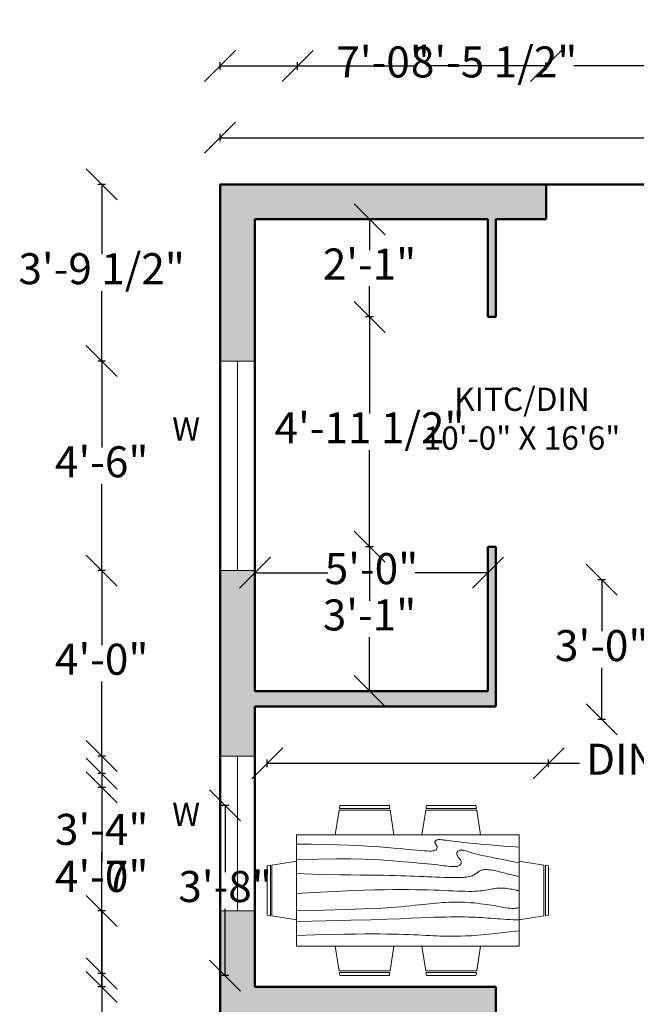
# Model space of a CAD drawing. Units: inches. Extents: x 3121 to 3511, y 1323 to 1998.
# Tile 9 of 10: x 3138 to 3297, y 1744 to 1998. Entities that reach past the tile are written whole.
import ezdxf

# ---------------------------------------------------------------- set-up
doc = ezdxf.new("R2010")
doc.units = ezdxf.units.IN
for name, color, linetype, lineweight in [('A-ANNO-DIMS', 2, 'Continuous', 18), ('A-ANNO-TEXT', 7, 'Continuous', 18), ('A-AREA-IDEN', 7, 'Continuous', 25), ('A-FURN', 8, 'Continuous', 18), ('A-GLAZ', 4, 'Continuous', 18), ('A-WALL', 7, 'Continuous', 50), ('A-WALL-PATT', 3, 'Continuous', 13)]:
    doc.layers.add(name, color=color, linetype=linetype, lineweight=lineweight)
doc.styles.get("Standard").update_dxf_attribs({"font": 'arial.ttf'})
doc.dimstyles.new('ISO-25', dxfattribs={"dimtxt": 8, "dimasz": 8, "dimexe": 1, "dimexo": 1, "dimtad": 0, "dimtih": 1, "dimtoh": 1, "dimlunit": 3, "dimtxsty": 'Standard', "dimblk": 'OBLIQUE', "dimcen": 2.5, "dimclrt": 1, "dimadec": 0, "dimazin": 0, "dimtfac": 1, "dimtmove": 0, "dimatfit": 3, "dimfxl": 1, "dimfxlon": 1, "dimarcsym": 0})

# ---------------------------------------------------------------- blocks, each defined once
blk = doc.blocks.new('Dining Set - 36 x 72 in.')
for p, q in [((-22.2343, 26.00059), (-23.4847, 17.99762)), ((-22.2304, 26), (-5.7608, 26)), ((-22, 27.5), (-22.1562, 26.50042)), ((-5.8416, 26.5), (-22.1534, 26.5)), ((-22, 27.5), (-6, 27.5)), ((-5.8437, 26.49966), (-6, 27.5)), ((-4.5152, 17.99762), (-5.7655, 25.99926)), ((5.7657, 26.00059), (4.5153, 17.99762)), ((5.7696, 26), (22.2392, 26)), ((6, 27.5), (5.8438, 26.50042)), ((22.1584, 26.5), (5.8466, 26.5)), ((6, 27.5), (22, 27.5)), ((22.1563, 26.49966), (22, 27.5)), ((23.4848, 17.99762), (22.2345, 25.99926)), ((36, 18), (-36, 18)), ((-36, 18), (-36, -18)), ((36, -18), (36, 18)), ((-45.5, 8), (-44.5004, 8.15617)), ((-45.5, 8), (-45.5, -8)), ((-44.5, -8.15843), (-44.5, 8.15338)), ((-44.0006, 8.23428), (-35.9976, 9.48474)), ((-44, 8.23041), (-44, -8.23915)), ((44.0006, 8.23428), (35.9976, 9.48474)), ((44, 8.23041), (44, -8.23915)), ((44.5, -8.15843), (44.5, 8.15338)), ((45.5, 8), (44.5005, 8.15617)), ((45.5, 8), (45.5, -8)), ((-44.4997, -8.15631), (-45.5, -8)), ((-35.9976, -9.48476), (-43.9993, -8.2345)), ((35.9976, -9.48476), (43.9993, -8.2345)), ((44.4997, -8.15631), (45.5, -8)), ((-36, -18), (36, -18)), ((-22.2343, -26.0006), (-23.4847, -17.99762)), ((-4.5152, -17.99762), (-5.7655, -25.99928)), ((5.7657, -26.0006), (4.5153, -17.99762)), ((23.4848, -17.99762), (22.2345, -25.99928)), ((-22.2304, -26), (-5.7608, -26)), ((-22, -27.5), (-22.1562, -26.50044)), ((-5.8416, -26.5), (-22.1534, -26.5)), ((-22, -27.5), (-6, -27.5)), ((-5.8437, -26.49967), (-6, -27.5)), ((5.7696, -26), (22.2392, -26)), ((6, -27.5), (5.8438, -26.50044)), ((22.1584, -26.5), (5.8466, -26.5)), ((6, -27.5), (22, -27.5)), ((22.1563, -26.49967), (22, -27.5))]:
    blk.add_line(p, q)
for points in [[(-36, 15), (-31.1772, 14.97754), (-26.8079, 14.91406), (-22.8538, 14.81543), (-19.276, 14.6875), (-16.0362, 14.53613), (-13.0957, 14.36718), (-10.4159, 14.18652), (-7.9583, 14), (-5.6904, 13.81315), (-3.6035, 13.63021), (-1.6954, 13.45508), (0.0365, 13.29166), (1.5945, 13.14388), (2.9811, 13.01562), (4.1988, 12.9108), (5.25, 12.83333), (6.1393, 12.78613), (6.8802, 12.76823), (7.4883, 12.77767), (7.9792, 12.8125), (8.3685, 12.87077), (8.6719, 12.95052), (8.9049, 13.0498), (9.0833, 13.16666), (9.2205, 13.29899), (9.3216, 13.44401), (9.3895, 13.59879), (9.4271, 13.76041), (9.4373, 13.92594), (9.4232, 14.09245), (9.3875, 14.257), (9.3333, 14.41666), (9.2638, 14.56917), (9.1836, 14.71484), (9.0975, 14.85465), (9.0104, 14.98958), (8.9272, 15.1206), (8.8529, 15.2487), (8.7922, 15.37483), (8.75, 15.5), (8.7305, 15.62467), (8.7344, 15.74739), (8.7617, 15.86621), (8.8125, 15.97916), (8.8867, 16.08431), (8.9844, 16.17968), (9.1055, 16.26334), (9.25, 16.33333), (9.4189, 16.38802), (9.6172, 16.42708), (9.8506, 16.45052), (10.125, 16.45833), (10.4463, 16.45052), (10.8203, 16.42708), (11.2529, 16.38802), (11.75, 16.33333), (12.3184, 16.26318), (12.9694, 16.17838), (13.7151, 16.07991), (14.5677, 15.96875), (15.5395, 15.84586), (16.6426, 15.71224), (17.8893, 15.56884), (19.2917, 15.41666), (20.859, 15.25667), (22.5879, 15.08984), (24.4721, 14.91715), (26.5052, 14.73958), (28.6809, 14.5581), (30.9929, 14.3737), (33.4347, 14.18733), (36, 14)], [(-36, 10), (-28.9766, 10.14274), (-23.1725, 10.20442), (-18.4241, 10.19775), (-14.5677, 10.13541), (-11.4399, 10.03011), (-8.877, 9.89453), (-6.7154, 9.74137), (-4.7917, 9.58333), (-2.9698, 9.43082), (-1.2246, 9.28515), (0.4415, 9.14534), (2.026, 9.01041), (3.5266, 8.87939), (4.9408, 8.7513), (6.266, 8.62516), (7.5, 8.5), (8.6411, 8.37549), (9.6914, 8.2539), (10.6538, 8.13818), (11.5312, 8.03125), (12.3267, 7.93603), (13.043, 7.85547), (13.6831, 7.79248), (14.25, 7.75), (14.7471, 7.7303), (15.1797, 7.73307), (15.5537, 7.75732), (15.875, 7.80208), (16.1494, 7.86637), (16.3828, 7.94922), (16.5811, 8.04964), (16.75, 8.16666), (16.8944, 8.29915), (17.0143, 8.44531), (17.1089, 8.60319), (17.1771, 8.77083), (17.218, 8.94629), (17.2305, 9.1276), (17.2137, 9.31282), (17.1667, 9.5), (17.0895, 9.6875), (16.987, 9.875), (16.8649, 10.0625), (16.7292, 10.25), (16.5856, 10.4375), (16.4401, 10.625), (16.2985, 10.8125), (16.1667, 11), (16.05, 11.18733), (15.9518, 11.3737), (15.8752, 11.5581), (15.8229, 11.73958), (15.798, 11.91715), (15.8034, 12.08984), (15.842, 12.25667), (15.9167, 12.41666), (16.0295, 12.56836), (16.1784, 12.70833), (16.3605, 12.83268), (16.5729, 12.9375), (16.8127, 13.01888), (17.0768, 13.07291), (17.3625, 13.0957), (17.6667, 13.08333), (17.9894, 13.03312), (18.3418, 12.94726), (18.7382, 12.82918), (19.1927, 12.68229), (19.7195, 12.51001), (20.3327, 12.31575), (21.0465, 12.10294), (21.875, 11.875), (22.8357, 11.63354), (23.959, 11.37304), (25.2786, 11.08618), (26.8282, 10.76562), (28.6414, 10.40405), (30.752, 9.99414), (33.1936, 9.52856), (36, 9)], [(-36, 5.5), (-30.7157, 5.3348), (-26.069, 5.20963), (-21.9946, 5.11767), (-18.4271, 5.05208), (-15.3009, 5.00602), (-12.5508, 4.97265), (-10.1112, 4.94515), (-7.9167, 4.91666), (-5.909, 4.88167), (-4.0586, 4.83984), (-2.3429, 4.79215), (-0.7396, 4.73958), (0.7739, 4.6831), (2.22, 4.6237), (3.6213, 4.56233), (5, 4.5), (6.373, 4.43782), (7.7344, 4.3776), (9.0723, 4.32129), (10.375, 4.27083), (11.6309, 4.22819), (12.8281, 4.19531), (13.9551, 4.17415), (15, 4.16666), (15.954, 4.17448), (16.819, 4.19791), (17.6001, 4.23698), (18.3021, 4.29166), (18.9299, 4.36198), (19.4883, 4.44791), (19.9823, 4.54948), (20.4167, 4.66666), (20.7969, 4.79899), (21.1302, 4.94401), (21.4245, 5.09879), (21.6875, 5.26041), (21.9271, 5.42594), (22.1511, 5.59245), (22.3672, 5.757), (22.5834, 5.91666), (22.8065, 6.06868), (23.0404, 6.21093), (23.2879, 6.34147), (23.5521, 6.45833), (23.8358, 6.55957), (24.142, 6.64323), (24.4735, 6.70735), (24.8334, 6.75), (25.2235, 6.76969), (25.642, 6.76692), (26.0858, 6.74267), (26.5521, 6.69791), (27.0379, 6.63362), (27.5404, 6.55078), (28.0565, 6.45036), (28.5834, 6.33333), (29.1242, 6.19987), (29.7071, 6.04687), (30.3661, 5.87044), (31.1354, 5.66666), (32.0493, 5.43164), (33.142, 5.16146), (34.4475, 4.85221), (36, 4.5)], [(-36, -1), (-30.7915, -0.6591), (-26.0195, -0.38216), (-21.6519, -0.16284), (-17.6563, 0.00521), (-14.0005, 0.12833), (-10.6523, 0.21289), (-7.5796, 0.26522), (-4.75, 0.29166), (-2.134, 0.29793), (0.2878, 0.28711), (2.5317, 0.26163), (4.6146, 0.22396), (6.5529, 0.17651), (8.3633, 0.12174), (10.0623, 0.06209), (11.6667, 0), (13.1899, -0.06201), (14.6341, -0.1211), (15.9982, -0.17432), (17.2813, -0.21875), (18.4823, -0.25147), (19.6003, -0.26953), (20.6343, -0.27002), (21.5834, -0.25), (22.4481, -0.20768), (23.2357, -0.14584), (23.9549, -0.06836), (24.6146, 0.02083), (25.2235, 0.11784), (25.7904, 0.21875), (26.3241, 0.31966), (26.8334, 0.41666), (27.3265, 0.50618), (27.8099, 0.58593), (28.2894, 0.65397), (28.7709, 0.70833), (29.2601, 0.74707), (29.763, 0.76823), (30.2855, 0.76985), (30.8334, 0.75), (31.4088, 0.70784), (31.9994, 0.64713), (32.589, 0.57275), (33.1615, 0.48958), (33.7008, 0.4025), (34.1908, 0.3164), (34.6153, 0.23616), (34.9584, 0.16666), (35.2099, 0.11165), (35.3848, 0.07031), (35.504, 0.04069), (35.5886, 0.02083), (35.6594, 0.00879), (35.7377, 0.0026), (35.8442, 0.00032), (36, 0)], [(-36, -6.5), (-27.1843, -6.31267), (-20.084, -6.1263), (-14.469, -5.9419), (-10.1094, -5.76042), (-6.7752, -5.58285), (-4.2363, -5.41016), (-2.2629, -5.24333), (-0.625, -5.08334), (0.8708, -4.93099), (2.2715, -4.78646), (3.5872, -4.64974), (4.8281, -4.52084), (6.0046, -4.39974), (7.127, -4.28646), (8.2053, -4.18099), (9.25, -4.08334), (10.2705, -3.99382), (11.2734, -3.91407), (12.2647, -3.84603), (13.25, -3.79167), (14.2354, -3.75293), (15.2266, -3.73177), (16.2295, -3.73015), (17.25, -3.75), (18.2912, -3.79248), (19.3451, -3.85547), (20.4009, -3.93604), (21.4479, -4.03125), (22.4754, -4.13819), (23.4727, -4.25391), (24.4289, -4.37549), (25.3334, -4.5), (26.1785, -4.62492), (26.9694, -4.74935), (27.7145, -4.87281), (28.4219, -4.99479), (29.1, -5.11483), (29.7572, -5.23242), (30.4016, -5.34709), (31.0417, -5.45834), (31.6837, -5.56437), (32.3262, -5.65821), (32.9658, -5.73153), (33.599, -5.77604), (34.2224, -5.78345), (34.8327, -5.74545), (35.4264, -5.65373), (36, -5.5)], [(-36, -10), (-26.4022, -9.81299), (-18.4675, -9.62891), (-11.9839, -9.45069), (-6.7396, -9.28125), (-2.5226, -9.12354), (0.8789, -8.98047), (3.6769, -8.85498), (6.0833, -8.75), (8.2767, -8.66765), (10.3021, -8.60677), (12.1712, -8.56543), (13.8958, -8.54167), (15.4876, -8.53353), (16.9583, -8.53907), (18.3197, -8.55632), (19.5834, -8.58334), (20.7616, -8.61841), (21.8685, -8.66081), (22.9188, -8.71004), (23.9271, -8.76563), (24.9081, -8.82707), (25.8763, -8.89388), (26.8465, -8.96558), (27.8334, -9.04167), (28.8474, -9.12118), (29.8828, -9.20117), (30.93, -9.27824), (31.9792, -9.34896), (33.0205, -9.40991), (34.0443, -9.45768), (35.0407, -9.48885), (36, -9.5)], [(-36, -14.5), (-30.0881, -14.33513), (-25.0332, -14.21224), (-20.7312, -14.12647), (-17.0781, -14.07292), (-13.97, -14.04671), (-11.3027, -14.04297), (-8.9724, -14.05681), (-6.875, -14.08334), (-4.9224, -14.11833), (-3.0905, -14.16016), (-1.3709, -14.20785), (0.2448, -14.26042), (1.7647, -14.3169), (3.1973, -14.3763), (4.5507, -14.43767), (5.8333, -14.5), (7.0554, -14.5621), (8.235, -14.62175), (9.3922, -14.67652), (10.5469, -14.72396), (11.7192, -14.76164), (12.929, -14.78711), (14.1965, -14.79794), (15.5417, -14.79167), (16.9933, -14.76424), (18.6152, -14.70508), (20.4804, -14.60197), (22.6615, -14.44271), (25.2312, -14.21509), (28.2624, -13.9069), (31.8277, -13.50594), (36, -13)]]:
    blk.add_lwpolyline(points)
blk = doc.blocks.new('_Oblique')
at = {"color": 0, "linetype": 'ByBlock', "lineweight": -2}
blk.add_line((-0.5, -0.5), (0.5, 0.5), dxfattribs=at)
blk = doc.blocks.new('*D17')
at = {"layer": 'A-ANNO-DIMS', "color": 0, "lineweight": -2, "transparency": 16777216}
for p, q in [((3189.92, 1966.81), (3189.92, 1968.81)), ((3456.92, 1966.81), (3456.92, 1968.81)), ((3189.92, 1967.81), (3308.98, 1967.81)), ((3456.92, 1967.81), (3337.85, 1967.81))]:
    blk.add_line(p, q, dxfattribs=at)
at = {"layer": 'Defpoints', "color": 0, "transparency": 16777216}
for p in [(3456.92, 1967.81), (3189.92, 1955.78), (3456.92, 1955.78)]:
    blk.add_point(p, dxfattribs=at)
at = {"layer": 'A-ANNO-DIMS', "color": 0, "lineweight": -2, "transparency": 16777216, "xscale": 8, "yscale": 8, "zscale": 8, "rotation": 180}
blk.add_blockref('_Oblique', (3189.92, 1967.81), dxfattribs=at)
at = {"layer": 'A-ANNO-DIMS', "color": 0, "lineweight": -2, "transparency": 16777216, "xscale": 8, "yscale": 8, "zscale": 8}
blk.add_blockref('_Oblique', (3456.92, 1967.81), dxfattribs=at)
at = {"layer": 'A-ANNO-DIMS', "color": 0, "transparency": 16777216, "insert": (3323.42, 1967.81), "char_height": 8, "attachment_point": 5}
blk.add_mtext('22\'-3"', dxfattribs=at)
blk = doc.blocks.new('*D27')
at = {"layer": 'A-ANNO-DIMS', "color": 0, "lineweight": -2, "transparency": 16777216}
for p, q in [((3202.09, 1805.46), (3202.09, 1807.46)), ((3202.09, 1806.46), (3274.67, 1806.46)), ((3274.67, 1805.46), (3274.67, 1807.46)), ((3274.67, 1806.46), (3282.67, 1806.46))]:
    blk.add_line(p, q, dxfattribs=at)
at = {"layer": 'Defpoints', "color": 0, "transparency": 16777216}
for p in [(3274.67, 1806.46), (3202.09, 1795.57), (3274.67, 1795.57)]:
    blk.add_point(p, dxfattribs=at)
at = {"layer": 'A-ANNO-DIMS', "color": 0, "lineweight": -2, "transparency": 16777216, "xscale": 8, "yscale": 8, "zscale": 8, "rotation": 180}
blk.add_blockref('_Oblique', (3202.09, 1806.46), dxfattribs=at)
at = {"layer": 'A-ANNO-DIMS', "color": 0, "lineweight": -2, "transparency": 16777216, "xscale": 8, "yscale": 8, "zscale": 8}
blk.add_blockref('_Oblique', (3274.67, 1806.46), dxfattribs=at)
at = {"layer": 'A-ANNO-DIMS', "color": 1, "transparency": 16777216, "insert": (3336.58, 1806.46), "char_height": 8, "attachment_point": 5}
blk.add_mtext('DINING SET 6\'-0 1/2"', dxfattribs=at)
blk = doc.blocks.new('*D28')
at = {"layer": 'A-ANNO-DIMS', "color": 0, "lineweight": -2, "transparency": 16777216}
for p, q in [((3192.2, 1795.57), (3190.2, 1795.57)), ((3191.2, 1795.57), (3191.2, 1778.35)), ((3191.2, 1751.7), (3191.2, 1768.92)), ((3192.2, 1751.7), (3190.2, 1751.7))]:
    blk.add_line(p, q, dxfattribs=at)
at = {"layer": 'Defpoints', "color": 0, "transparency": 16777216}
for p in [(3191.2, 1795.57), (3202.09, 1795.57), (3202.09, 1751.7)]:
    blk.add_point(p, dxfattribs=at)
at = {"layer": 'A-ANNO-DIMS', "color": 0, "lineweight": -2, "transparency": 16777216, "xscale": 8, "yscale": 8, "zscale": 8}
for p, rotation in [((3191.2, 1795.57), 90), ((3191.2, 1751.7), 270)]:
    blk.add_blockref('_Oblique', p, dxfattribs=dict(at, rotation=rotation))
at = {"layer": 'A-ANNO-DIMS', "color": 1, "transparency": 16777216, "insert": (3191.2, 1773.63), "char_height": 8, "attachment_point": 5}
blk.add_mtext('3\'-8"', dxfattribs=at)
blk = doc.blocks.new('*D39')
at = {"layer": 'A-ANNO-DIMS', "color": 0, "lineweight": -2, "transparency": 16777216}
for p, q in [((3160.37, 1768.39), (3158.37, 1768.39)), ((3159.37, 1768.39), (3159.37, 1735.04)), ((3159.37, 1692.28), (3159.37, 1725.62)), ((3160.37, 1692.28), (3158.37, 1692.28))]:
    blk.add_line(p, q, dxfattribs=at)
at = {"layer": 'Defpoints', "color": 0, "transparency": 16777216}
for p in [(3159.37, 1768.39), (3189.92, 1768.39), (3189.92, 1692.28)]:
    blk.add_point(p, dxfattribs=at)
at = {"layer": 'A-ANNO-DIMS', "color": 0, "lineweight": -2, "transparency": 16777216, "xscale": 8, "yscale": 8, "zscale": 8}
for p, rotation in [((3159.37, 1768.39), 90), ((3159.37, 1692.28), 270)]:
    blk.add_blockref('_Oblique', p, dxfattribs=dict(at, rotation=rotation))
at = {"layer": 'A-ANNO-DIMS', "color": 1, "transparency": 16777216, "insert": (3159.37, 1730.33), "char_height": 8, "attachment_point": 5}
blk.add_mtext('6\'-4"', dxfattribs=at)
blk = doc.blocks.new('*D40')
at = {"layer": 'A-ANNO-DIMS', "color": 0, "lineweight": -2, "transparency": 16777216}
for p, q in [((3160.37, 1808.33), (3158.37, 1808.33)), ((3159.37, 1808.33), (3159.37, 1793.07)), ((3159.37, 1768.39), (3159.37, 1783.65)), ((3160.37, 1768.39), (3158.37, 1768.39))]:
    blk.add_line(p, q, dxfattribs=at)
at = {"layer": 'Defpoints', "color": 0, "transparency": 16777216}
for p in [(3159.37, 1808.33), (3189.92, 1808.33), (3189.92, 1768.39)]:
    blk.add_point(p, dxfattribs=at)
at = {"layer": 'A-ANNO-DIMS', "color": 0, "lineweight": -2, "transparency": 16777216, "xscale": 8, "yscale": 8, "zscale": 8}
for p, rotation in [((3159.37, 1808.33), 90), ((3159.37, 1768.39), 270)]:
    blk.add_blockref('_Oblique', p, dxfattribs=dict(at, rotation=rotation))
at = {"layer": 'A-ANNO-DIMS', "color": 1, "transparency": 16777216, "insert": (3159.37, 1788.36), "char_height": 8, "attachment_point": 5}
blk.add_mtext('3\'-4"', dxfattribs=at)
blk = doc.blocks.new('*D41')
at = {"layer": 'A-ANNO-DIMS', "color": 0, "lineweight": -2, "transparency": 16777216}
for p, q in [((3160.37, 1856.17), (3158.37, 1856.17)), ((3159.37, 1856.17), (3159.37, 1836.96)), ((3159.37, 1808.33), (3159.37, 1827.54)), ((3160.37, 1808.33), (3158.37, 1808.33))]:
    blk.add_line(p, q, dxfattribs=at)
at = {"layer": 'Defpoints', "color": 0, "transparency": 16777216}
for p in [(3159.37, 1856.17), (3189.92, 1856.17), (3189.92, 1808.33)]:
    blk.add_point(p, dxfattribs=at)
at = {"layer": 'A-ANNO-DIMS', "color": 0, "lineweight": -2, "transparency": 16777216, "xscale": 8, "yscale": 8, "zscale": 8}
for p, rotation in [((3159.37, 1856.17), 90), ((3159.37, 1808.33), 270)]:
    blk.add_blockref('_Oblique', p, dxfattribs=dict(at, rotation=rotation))
at = {"layer": 'A-ANNO-DIMS', "color": 1, "transparency": 16777216, "insert": (3159.37, 1832.25), "char_height": 8, "attachment_point": 5}
blk.add_mtext('4\'-0"', dxfattribs=at)
blk = doc.blocks.new('*D42')
at = {"layer": 'A-ANNO-DIMS', "color": 0, "lineweight": -2, "transparency": 16777216}
for p, q in [((3160.37, 1910.22), (3158.37, 1910.22)), ((3159.37, 1910.22), (3159.37, 1887.9)), ((3159.37, 1856.17), (3159.37, 1878.49)), ((3160.37, 1856.17), (3158.37, 1856.17))]:
    blk.add_line(p, q, dxfattribs=at)
at = {"layer": 'Defpoints', "color": 0, "transparency": 16777216}
for p in [(3159.37, 1910.22), (3189.92, 1910.22), (3189.92, 1856.17)]:
    blk.add_point(p, dxfattribs=at)
at = {"layer": 'A-ANNO-DIMS', "color": 0, "lineweight": -2, "transparency": 16777216, "xscale": 8, "yscale": 8, "zscale": 8}
for p, rotation in [((3159.37, 1910.22), 90), ((3159.37, 1856.17), 270)]:
    blk.add_blockref('_Oblique', p, dxfattribs=dict(at, rotation=rotation))
at = {"layer": 'A-ANNO-DIMS', "color": 1, "transparency": 16777216, "insert": (3159.37, 1883.19), "char_height": 8, "attachment_point": 5}
blk.add_mtext('4\'-6"', dxfattribs=at)
blk = doc.blocks.new('*D43')
at = {"layer": 'A-ANNO-DIMS', "color": 0, "lineweight": -2, "transparency": 16777216}
for p, q in [((3160.37, 1955.78), (3158.37, 1955.78)), ((3159.37, 1955.78), (3159.37, 1937.77)), ((3159.37, 1910.22), (3159.37, 1928.24)), ((3160.37, 1910.22), (3158.37, 1910.22))]:
    blk.add_line(p, q, dxfattribs=at)
at = {"layer": 'Defpoints', "color": 0, "transparency": 16777216}
for p in [(3159.37, 1955.78), (3189.92, 1955.78), (3189.92, 1910.22)]:
    blk.add_point(p, dxfattribs=at)
at = {"layer": 'A-ANNO-DIMS', "color": 0, "lineweight": -2, "transparency": 16777216, "xscale": 8, "yscale": 8, "zscale": 8}
for p, rotation in [((3159.37, 1955.78), 90), ((3159.37, 1910.22), 270)]:
    blk.add_blockref('_Oblique', p, dxfattribs=dict(at, rotation=rotation))
at = {"layer": 'A-ANNO-DIMS', "color": 1, "transparency": 16777216, "insert": (3159.37, 1933), "char_height": 8, "attachment_point": 5}
blk.add_mtext('3\'-9 1/2"', dxfattribs=at)
blk = doc.blocks.new('*D52')
at = {"layer": 'A-ANNO-DIMS', "color": 0, "lineweight": -2, "transparency": 16777216}
for p, q in [((3189.92, 1985.33), (3189.92, 1987.33)), ((3189.92, 1986.33), (3220.75, 1986.33)), ((3274.02, 1986.33), (3243.2, 1986.33)), ((3274.02, 1985.33), (3274.02, 1987.33))]:
    blk.add_line(p, q, dxfattribs=at)
at = {"layer": 'Defpoints', "color": 0, "transparency": 16777216}
for p in [(3274.02, 1986.33), (3189.92, 1955.78), (3274.02, 1955.78)]:
    blk.add_point(p, dxfattribs=at)
at = {"layer": 'A-ANNO-DIMS', "color": 0, "lineweight": -2, "transparency": 16777216, "xscale": 8, "yscale": 8, "zscale": 8, "rotation": 180}
blk.add_blockref('_Oblique', (3189.92, 1986.33), dxfattribs=at)
at = {"layer": 'A-ANNO-DIMS', "color": 0, "lineweight": -2, "transparency": 16777216, "xscale": 8, "yscale": 8, "zscale": 8}
blk.add_blockref('_Oblique', (3274.02, 1986.33), dxfattribs=at)
at = {"layer": 'A-ANNO-DIMS', "color": 1, "transparency": 16777216, "insert": (3231.97, 1986.33), "char_height": 8, "attachment_point": 5}
blk.add_mtext('7\'-0"', dxfattribs=at)
blk = doc.blocks.new('*D53')
at = {"layer": 'A-ANNO-DIMS', "color": 0, "lineweight": -2, "transparency": 16777216}
for p, q in [((3274.02, 1336.37), (3274.02, 1334.37)), ((3310.02, 1336.37), (3310.02, 1334.37)), ((3274.02, 1335.37), (3280.77, 1335.37)), ((3310.02, 1335.37), (3303.28, 1335.37))]:
    blk.add_line(p, q, dxfattribs=at)
at = {"layer": 'Defpoints', "color": 0, "transparency": 16777216}
for p in [(3274.02, 1946.78), (3310.02, 1946.78), (3310.02, 1335.37)]:
    blk.add_point(p, dxfattribs=at)
at = {"layer": 'A-ANNO-DIMS', "color": 0, "lineweight": -2, "transparency": 16777216, "xscale": 8, "yscale": 8, "zscale": 8, "rotation": 180}
blk.add_blockref('_Oblique', (3274.02, 1335.37), dxfattribs=at)
at = {"layer": 'A-ANNO-DIMS', "color": 0, "lineweight": -2, "transparency": 16777216, "xscale": 8, "yscale": 8, "zscale": 8}
blk.add_blockref('_Oblique', (3310.02, 1335.37), dxfattribs=at)
at = {"layer": 'A-ANNO-DIMS', "color": 1, "transparency": 16777216, "insert": (3292.02, 1335.37), "char_height": 8, "attachment_point": 5}
blk.add_mtext('3\'-0"', dxfattribs=at)
blk = doc.blocks.new('*D58')
at = {"layer": 'A-ANNO-DIMS', "color": 0, "lineweight": -2, "transparency": 16777216}
for p, q in [((3209.89, 1985.33), (3209.89, 1987.33)), ((3209.89, 1986.33), (3240.03, 1986.33)), ((3311.33, 1986.33), (3281.19, 1986.33)), ((3311.33, 1985.33), (3311.33, 1987.33))]:
    blk.add_line(p, q, dxfattribs=at)
at = {"layer": 'Defpoints', "color": 0, "transparency": 16777216}
for p in [(3311.33, 1986.33), (3209.89, 1424.78), (3311.33, 1424.78)]:
    blk.add_point(p, dxfattribs=at)
at = {"layer": 'A-ANNO-DIMS', "color": 0, "lineweight": -2, "transparency": 16777216, "xscale": 8, "yscale": 8, "zscale": 8, "rotation": 180}
blk.add_blockref('_Oblique', (3209.89, 1986.33), dxfattribs=at)
at = {"layer": 'A-ANNO-DIMS', "color": 0, "lineweight": -2, "transparency": 16777216, "xscale": 8, "yscale": 8, "zscale": 8}
blk.add_blockref('_Oblique', (3311.33, 1986.33), dxfattribs=at)
at = {"layer": 'A-ANNO-DIMS', "color": 1, "transparency": 16777216, "insert": (3260.61, 1986.33), "char_height": 8, "attachment_point": 5}
blk.add_mtext('8\'-5 1/2"', dxfattribs=at)
blk = doc.blocks.new('*D60')
at = {"layer": 'A-ANNO-DIMS', "color": 0, "lineweight": -2, "transparency": 16777216}
for p, q in [((3160.368016, 1803.784138), (3158.368016, 1803.784138)), ((3159.368016, 1803.784138), (3159.368016, 1780.909138)), ((3159.368016, 1748.784138), (3159.368016, 1771.659138)), ((3160.368016, 1748.784138), (3158.368016, 1748.784138))]:
    blk.add_line(p, q, dxfattribs=at)
at = {"layer": 'Defpoints', "color": 0, "transparency": 16777216}
for p in [(3159.368016, 1803.784138), (3370.918016, 1803.784138), (3370.918016, 1748.784138)]:
    blk.add_point(p, dxfattribs=at)
at = {"layer": 'A-ANNO-DIMS', "color": 0, "lineweight": -2, "transparency": 16777216, "xscale": 8, "yscale": 8, "zscale": 8}
for p, rotation in [((3159.368016, 1803.784138), 90), ((3159.368016, 1748.784138), 270)]:
    blk.add_blockref('_Oblique', p, dxfattribs=dict(at, rotation=rotation))
at = {"layer": 'A-ANNO-DIMS', "color": 1, "transparency": 16777216, "insert": (3159.368016, 1776.284138), "char_height": 8, "attachment_point": 5}
blk.add_mtext('4\'-7"', dxfattribs=at)
blk = doc.blocks.new('*D62')
at = {"layer": 'A-ANNO-DIMS', "color": 0, "lineweight": -2, "transparency": 16777216}
for p, q in [((3160.37, 1800.22), (3158.37, 1800.22)), ((3159.37, 1800.22), (3159.37, 1780.93)), ((3159.37, 1752.23), (3159.37, 1771.52)), ((3160.37, 1752.23), (3158.37, 1752.23))]:
    blk.add_line(p, q, dxfattribs=at)
at = {"layer": 'Defpoints', "color": 0, "transparency": 16777216}
for p in [(3159.37, 1800.22), (3318.92, 1800.22), (3318.92, 1752.23)]:
    blk.add_point(p, dxfattribs=at)
at = {"layer": 'A-ANNO-DIMS', "color": 0, "lineweight": -2, "transparency": 16777216, "xscale": 8, "yscale": 8, "zscale": 8}
for p, rotation in [((3159.37, 1800.22), 90), ((3159.37, 1752.23), 270)]:
    blk.add_blockref('_Oblique', p, dxfattribs=dict(at, rotation=rotation))
at = {"layer": 'A-ANNO-DIMS', "color": 1, "transparency": 16777216, "insert": (3159.37, 1776.22), "char_height": 8, "attachment_point": 5}
blk.add_mtext('4\'-0"', dxfattribs=at)
blk = doc.blocks.new('*D78')
at = {"layer": 'A-ANNO-DIMS', "color": 0, "lineweight": -2, "transparency": 16777216}
for p, q in [((3289.37, 1853.78), (3287.37, 1853.78)), ((3288.37, 1853.78), (3288.37, 1840.5)), ((3288.37, 1817.78), (3288.37, 1831.07)), ((3289.37, 1817.78), (3287.37, 1817.78))]:
    blk.add_line(p, q, dxfattribs=at)
at = {"layer": 'Defpoints', "color": 0, "transparency": 16777216}
for p in [(3288.37, 1853.78), (3318.92, 1853.78), (3318.92, 1817.78)]:
    blk.add_point(p, dxfattribs=at)
at = {"layer": 'A-ANNO-DIMS', "color": 0, "lineweight": -2, "transparency": 16777216, "xscale": 8, "yscale": 8, "zscale": 8}
for p, rotation in [((3288.37, 1853.78), 90), ((3288.37, 1817.78), 270)]:
    blk.add_blockref('_Oblique', p, dxfattribs=dict(at, rotation=rotation))
at = {"layer": 'A-ANNO-DIMS', "color": 1, "transparency": 16777216, "insert": (3288.37, 1835.78), "char_height": 8, "attachment_point": 5}
blk.add_mtext('3\'-0"', dxfattribs=at)
blk = doc.blocks.new('*D79')
at = {"layer": 'A-ANNO-DIMS', "color": 0, "lineweight": -2, "transparency": 16777216}
for p, q in [((3198.92, 1854.62), (3198.92, 1856.62)), ((3259.02, 1854.62), (3259.02, 1856.62)), ((3198.92, 1855.62), (3217.71, 1855.62)), ((3259.02, 1855.62), (3240.23, 1855.62))]:
    blk.add_line(p, q, dxfattribs=at)
at = {"layer": 'Defpoints', "color": 0, "transparency": 16777216}
for p in [(3259.02, 1855.62), (3198.92, 1825.07), (3259.02, 1825.07)]:
    blk.add_point(p, dxfattribs=at)
at = {"layer": 'A-ANNO-DIMS', "color": 0, "lineweight": -2, "transparency": 16777216, "xscale": 8, "yscale": 8, "zscale": 8, "rotation": 180}
blk.add_blockref('_Oblique', (3198.92, 1855.62), dxfattribs=at)
at = {"layer": 'A-ANNO-DIMS', "color": 0, "lineweight": -2, "transparency": 16777216, "xscale": 8, "yscale": 8, "zscale": 8}
blk.add_blockref('_Oblique', (3259.02, 1855.62), dxfattribs=at)
at = {"layer": 'A-ANNO-DIMS', "color": 1, "transparency": 16777216, "insert": (3228.97, 1855.62), "char_height": 8, "attachment_point": 5}
blk.add_mtext('5\'-0"', dxfattribs=at)
blk = doc.blocks.new('*D80')
at = {"layer": 'A-ANNO-DIMS', "color": 0, "lineweight": -2, "transparency": 16777216}
for p, q in [((3229.47, 1946.78), (3227.47, 1946.78)), ((3228.47, 1946.78), (3228.47, 1938.84)), ((3228.47, 1921.61), (3228.47, 1929.56)), ((3229.47, 1921.61), (3227.47, 1921.61))]:
    blk.add_line(p, q, dxfattribs=at)
at = {"layer": 'Defpoints', "color": 0, "transparency": 16777216}
for p in [(3228.47, 1946.78), (3259.02, 1946.78), (3259.02, 1921.61)]:
    blk.add_point(p, dxfattribs=at)
at = {"layer": 'A-ANNO-DIMS', "color": 0, "lineweight": -2, "transparency": 16777216, "xscale": 8, "yscale": 8, "zscale": 8}
for p, rotation in [((3228.47, 1946.78), 90), ((3228.47, 1921.61), 270)]:
    blk.add_blockref('_Oblique', p, dxfattribs=dict(at, rotation=rotation))
at = {"layer": 'A-ANNO-DIMS', "color": 1, "transparency": 16777216, "insert": (3228.47, 1934.2), "char_height": 8, "attachment_point": 5}
blk.add_mtext('2\'-1"', dxfattribs=at)
blk = doc.blocks.new('*D81')
at = {"layer": 'A-ANNO-DIMS', "color": 0, "lineweight": -2, "transparency": 16777216}
for p, q in [((3229.47, 1862.31), (3227.47, 1862.31)), ((3228.47, 1862.31), (3228.47, 1848.4)), ((3228.47, 1825.07), (3228.47, 1838.98)), ((3229.47, 1825.07), (3227.47, 1825.07))]:
    blk.add_line(p, q, dxfattribs=at)
at = {"layer": 'Defpoints', "color": 0, "transparency": 16777216}
for p in [(3228.47, 1862.31), (3259.02, 1862.31), (3259.02, 1825.07)]:
    blk.add_point(p, dxfattribs=at)
at = {"layer": 'A-ANNO-DIMS', "color": 0, "lineweight": -2, "transparency": 16777216, "xscale": 8, "yscale": 8, "zscale": 8}
for p, rotation in [((3228.47, 1862.31), 90), ((3228.47, 1825.07), 270)]:
    blk.add_blockref('_Oblique', p, dxfattribs=dict(at, rotation=rotation))
at = {"layer": 'A-ANNO-DIMS', "color": 1, "transparency": 16777216, "insert": (3228.47, 1843.69), "char_height": 8, "attachment_point": 5}
blk.add_mtext('3\'-1"', dxfattribs=at)
blk = doc.blocks.new('*D82')
at = {"layer": 'A-ANNO-DIMS', "color": 0, "lineweight": -2, "transparency": 16777216}
for p, q in [((3229.47, 1921.61), (3227.47, 1921.61)), ((3228.47, 1921.61), (3228.47, 1896.72)), ((3228.47, 1862.31), (3228.47, 1887.2)), ((3229.47, 1862.31), (3227.47, 1862.31))]:
    blk.add_line(p, q, dxfattribs=at)
at = {"layer": 'Defpoints', "color": 0, "transparency": 16777216}
for p in [(3228.47, 1921.61), (3259.02, 1921.61), (3259.02, 1862.31)]:
    blk.add_point(p, dxfattribs=at)
at = {"layer": 'A-ANNO-DIMS', "color": 0, "lineweight": -2, "transparency": 16777216, "xscale": 8, "yscale": 8, "zscale": 8}
for p, rotation in [((3228.47, 1921.61), 90), ((3228.47, 1862.31), 270)]:
    blk.add_blockref('_Oblique', p, dxfattribs=dict(at, rotation=rotation))
at = {"layer": 'A-ANNO-DIMS', "color": 1, "transparency": 16777216, "insert": (3228.47, 1891.96), "char_height": 8, "attachment_point": 5}
blk.add_mtext('4\'-11 1/2"', dxfattribs=at)

msp = doc.modelspace()

# ---------------------------------------------------------------- hatches: boundary and pattern name
at = {"layer": 'A-WALL-PATT'}
h = msp.add_hatch(color=256, dxfattribs=at)
h.dxf.hatch_style = 1
h.paths.add_polyline_path([(3274.023, 1955.784), (3189.918, 1955.784), (3189.918, 1910.219), (3198.918, 1910.219), (3198.918, 1946.784), (3259.023, 1946.784), (3259.023, 1921.61), (3261.023, 1921.61), (3261.023, 1946.784), (3274.023, 1946.784)])
h.paths.add_polyline_path([(3327.918, 1946.784), (3334.156, 1946.784), (3334.156, 1955.784), (3310.023, 1955.784), (3310.023, 1946.784), (3318.918, 1946.784), (3318.918, 1929.796), (3311.644, 1929.796), (3311.644, 1927.007), (3324.033, 1927.007), (3324.033, 1871.381), (3311.644, 1871.381), (3311.644, 1868.381), (3318.918, 1868.381), (3318.918, 1853.784), (3327.918, 1853.784)])
h.paths.add_polyline_path([(3456.918, 1955.784), (3384.562, 1955.784), (3384.562, 1946.784), (3447.918, 1946.784), (3447.918, 1877.779), (3456.918, 1877.779)])
h.paths.add_polyline_path([(3456.918, 1835.782), (3447.918, 1835.782), (3447.918, 1814.784), (3414.918, 1814.784), (3414.918, 1803.784), (3447.918, 1803.784), (3447.918, 1793.443), (3456.918, 1793.443)])
h.paths.add_polyline_path([(3456.918, 1558.434), (3447.918, 1558.434), (3447.918, 1547.784), (3375.918, 1547.784), (3375.918, 1598.784), (3378.918, 1598.784), (3378.918, 1602.284), (3375.918, 1602.284), (3375.918, 1674.284), (3369.918, 1674.284), (3369.918, 1547.784), (3364.418, 1547.784), (3364.418, 1538.784), (3447.918, 1538.784), (3447.918, 1512.628), (3456.918, 1512.628)])
h.paths.add_polyline_path([(3456.918, 1460.558), (3447.918, 1460.558), (3447.918, 1424.784), (3412.543, 1424.784), (3412.543, 1415.784), (3456.918, 1415.784)])
h.paths.add_polyline_path([(3358.149, 1424.784), (3322.918, 1424.784), (3322.918, 1538.784), (3328.418, 1538.784), (3328.418, 1547.784), (3308.208, 1547.784), (3308.208, 1538.784), (3318.918, 1538.784), (3318.918, 1424.784), (3311.328, 1424.784), (3311.328, 1415.784), (3358.149, 1415.784)])
h.paths.add_polyline_path([(3207.562, 1547.784), (3198.918, 1547.784), (3198.918, 1607.327), (3189.918, 1607.327), (3189.918, 1513.073), (3198.918, 1513.073), (3198.918, 1538.784), (3207.562, 1538.784)])
h.paths.add_polyline_path([(3198.918, 1461.548), (3189.918, 1461.548), (3189.918, 1415.784), (3209.892, 1415.784), (3209.892, 1424.784), (3198.918, 1424.784)])
h.paths.add_polyline_path([(3272.208, 1547.784), (3238.766, 1547.784), (3238.766, 1538.784), (3272.208, 1538.784)])
h.paths.add_polyline_path([(3261.023, 1748.784), (3198.918, 1748.784), (3198.918, 1768.387), (3189.918, 1768.387), (3189.918, 1692.279), (3198.918, 1692.279), (3198.918, 1739.784), (3261.023, 1739.784)])
h.paths.add_polyline_path([(3198.918, 1856.171), (3189.918, 1856.171), (3189.918, 1808.331), (3198.918, 1808.331), (3198.918, 1821.074), (3261.023, 1821.074), (3261.023, 1862.309), (3259.023, 1862.309), (3259.023, 1825.074), (3198.918, 1825.074)])

# ---------------------------------------------------------------- linework, layer by layer
at = {"layer": 'A-GLAZ'}
for p, q in [((3198.918, 1910.219), (3189.918, 1910.219)), ((3194.418, 1856.171), (3194.418, 1910.219)), ((3198.918, 1856.171), (3189.918, 1856.171)), ((3198.918, 1808.331), (3189.918, 1808.331)), ((3194.418, 1808.331), (3194.418, 1768.387)), ((3189.918, 1768.387), (3198.918, 1768.387))]:
    msp.add_line(p, q, dxfattribs=at)
at = {"layer": 'A-WALL'}
for p, q in [((3456.918, 1955.784), (3189.918, 1955.784)), ((3189.918, 1955.784), (3189.918, 1415.784)), ((3274.023, 1946.784), (3274.023, 1955.784)), ((3198.918, 1946.784), (3198.918, 1825.074)), ((3259.023, 1946.784), (3198.918, 1946.784)), ((3259.023, 1921.61), (3259.023, 1946.784)), ((3261.023, 1921.61), (3261.023, 1946.784)), ((3274.023, 1946.784), (3261.023, 1946.784)), ((3259.023, 1921.61), (3261.023, 1921.61)), ((3259.023, 1825.074), (3259.023, 1862.309)), ((3259.023, 1862.309), (3261.023, 1862.309)), ((3261.023, 1821.074), (3261.023, 1862.309)), ((3198.918, 1825.074), (3259.023, 1825.074)), ((3198.918, 1821.074), (3261.023, 1821.074)), ((3198.918, 1821.074), (3198.918, 1748.784)), ((3261.023, 1748.784), (3198.918, 1748.784)), ((3261.023, 1748.784), (3261.023, 1739.784))]:
    msp.add_line(p, q, dxfattribs=at)

# ---------------------------------------------------------------- block references
at = {"layer": 'A-FURN', "xscale": 0.7976107073757374, "yscale": 0.7976107073757374, "zscale": 0.7976107073757374}
msp.add_blockref('Dining Set - 36 x 72 in.', (3238.376, 1773.635), dxfattribs=at)

# ---------------------------------------------------------------- texts
at = {"layer": 'A-ANNO-TEXT', "char_height": 6, "attachment_point": 1}
for insert in [(3174.942, 1895.703), (3174.942, 1796.295)]:
    msp.add_mtext_dynamic_manual_height_columns('\\pxqc;W', width=12.42925, gutter_width=12.5, heights=[0], dxfattribs=dict(at, insert=insert))
at = {"layer": 'A-AREA-IDEN', "insert": (3232.971, 1903.35), "char_height": 6, "attachment_point": 1}
msp.add_mtext_dynamic_manual_height_columns('\\pxqc;KITC/DIN\\P10\'-0" X 16\'6"', width=69.63762, gutter_width=12.5, heights=[0], dxfattribs=at)

# ---------------------------------------------------------------- dimensions: what is measured, and where the dimension line sits
at = {"layer": 'A-ANNO-DIMS'}
for base, p1, p2, override, picture, middle in [((3311.328, 1986.334), (3209.892, 1424.784), (3311.328, 1424.784), {"dimdec": 1, "dimlfac": 1, "dimrnd": 0, "dimzin": 1, "dimdsep": 46, "dimlunit": 4, "dimfrac": 2}, '*D58', (3260.61, 1986.334)), ((3274.023, 1986.334), (3189.918, 1955.784), (3274.023, 1955.784), {"dimdec": 1, "dimlfac": 1, "dimrnd": 0, "dimzin": 1, "dimdsep": 46, "dimlunit": 4, "dimfrac": 2}, '*D52', (3231.97, 1986.334)), ((3456.918, 1967.814), (3189.918, 1955.784), (3456.918, 1955.784), {"dimclrd": 0, "dimclre": 0, "dimclrt": 0}, '*D17', (3323.418, 1967.814)), ((3310.023, 1335.367), (3274.023, 1946.784), (3310.023, 1946.784), {"dimdec": 1, "dimlfac": 1, "dimrnd": 0, "dimzin": 1, "dimdsep": 46, "dimlunit": 4, "dimfrac": 2}, '*D53', (3292.023, 1335.367)), ((3259.023, 1855.624), (3198.918, 1825.074), (3259.023, 1825.074), {"dimdec": 1, "dimlfac": 1, "dimrnd": 0, "dimzin": 1, "dimdsep": 46, "dimlunit": 4, "dimfrac": 2}, '*D79', (3228.97, 1855.624))]:
    dim = msp.add_linear_dim(base=base, p1=p1, p2=p2, dimstyle='ISO-25', override=override, dxfattribs=at)
    dim.commit()
    dim.dimension.update_dxf_attribs({"geometry": picture, "text_midpoint": middle})
for base, p1, p2, picture, middle in [((3159.368, 1955.784), (3189.918, 1910.219), (3189.918, 1955.784), '*D43', (3159.368, 1933.001)), ((3228.473, 1946.784), (3259.023, 1921.61), (3259.023, 1946.784), '*D80', (3228.473, 1934.197)), ((3228.473, 1921.61), (3259.023, 1862.309), (3259.023, 1921.61), '*D82', (3228.473, 1891.959)), ((3159.368, 1910.219), (3189.918, 1856.171), (3189.918, 1910.219), '*D42', (3159.368, 1883.195)), ((3228.473, 1862.309), (3259.023, 1825.074), (3259.023, 1862.309), '*D81', (3228.473, 1843.692)), ((3159.368, 1856.171), (3189.918, 1808.331), (3189.918, 1856.171), '*D41', (3159.368, 1832.251)), ((3288.368, 1853.784), (3318.918, 1817.784), (3318.918, 1853.784), '*D78', (3288.368, 1835.784)), ((3159.368, 1808.331), (3189.918, 1768.387), (3189.918, 1808.331), '*D40', (3159.368, 1788.359)), ((3159.368, 1803.784), (3370.918, 1748.784), (3370.918, 1803.784), '*D60', (3159.368, 1776.284)), ((3159.368, 1800.224), (3318.918, 1752.226), (3318.918, 1800.224), '*D62', (3159.368, 1776.225)), ((3191.198, 1795.569), (3202.085, 1751.7), (3202.085, 1795.569), '*D28', (3191.198, 1773.635)), ((3159.368, 1768.387), (3189.918, 1692.279), (3189.918, 1768.387), '*D39', (3159.368, 1730.333))]:
    dim = msp.add_linear_dim(base=base, p1=p1, p2=p2, angle=90, dimstyle='ISO-25', override={"dimdec": 1, "dimlfac": 1, "dimrnd": 0, "dimzin": 1, "dimdsep": 46, "dimlunit": 4, "dimfrac": 2}, dxfattribs=at)
    dim.commit()
    dim.dimension.update_dxf_attribs({"geometry": picture, "text_midpoint": middle})
dim = msp.add_linear_dim(base=(3274.668, 1806.456), p1=(3202.085, 1795.569), p2=(3274.668, 1795.569), text='DINING SET <>', dimstyle='ISO-25', override={"dimdec": 1, "dimlfac": 1, "dimrnd": 0, "dimzin": 1, "dimdsep": 46, "dimlunit": 4, "dimfrac": 2}, dxfattribs=at)
dim.commit()
dim.dimension.update_dxf_attribs({"geometry": '*D27', "text_midpoint": (3336.578, 1806.456)})

doc.saveas('drawing.dxf')
